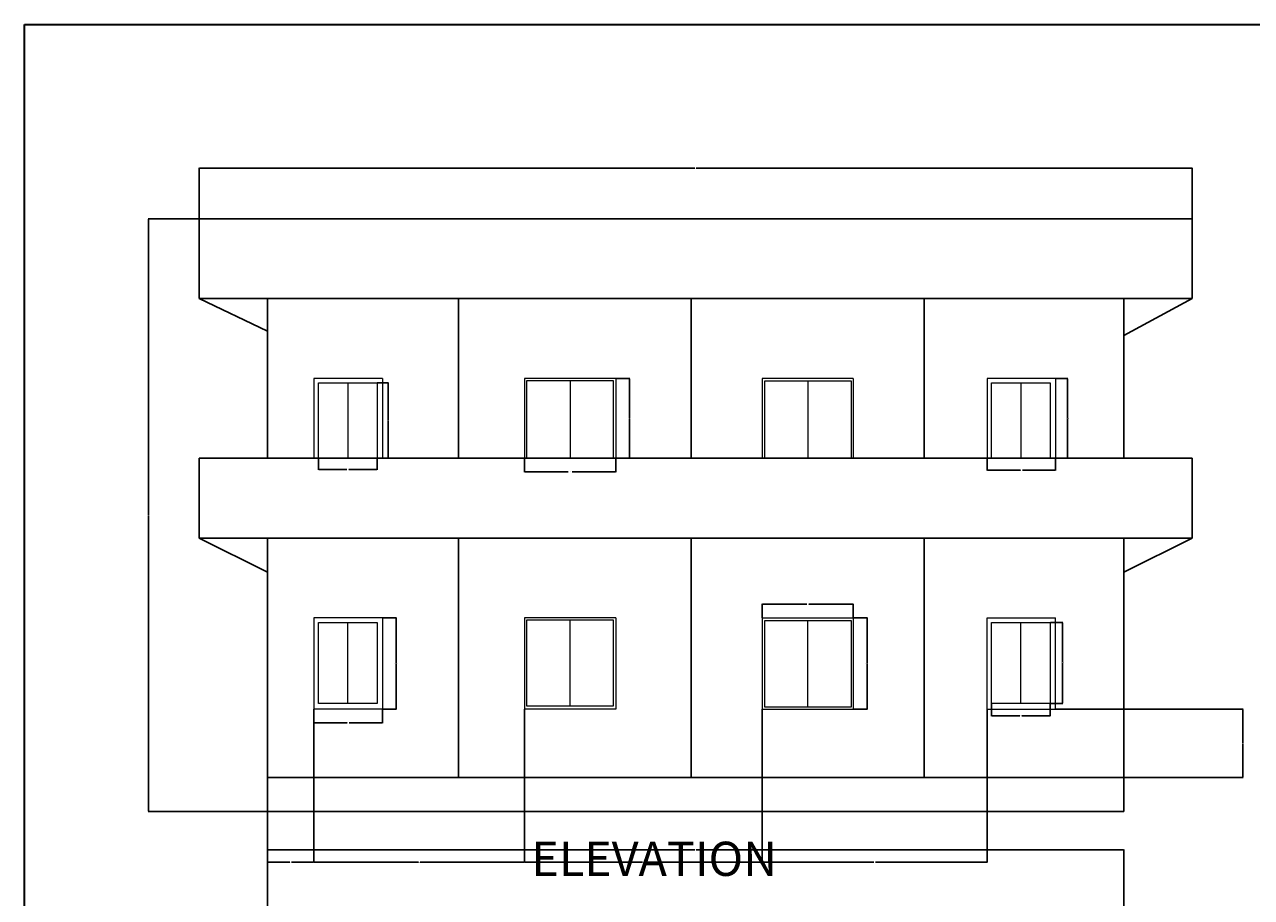
# Model space of a CAD drawing. Units: inches. Extents: x 2043 to 3387, y 1535 to 2797.
# Tile 3 of 7: x 2043 to 2688, y 2337 to 2797. Entities that reach past the tile are written whole.
import ezdxf

# ---------------------------------------------------------------- set-up
doc = ezdxf.new("R2010")
doc.units = ezdxf.units.IN
for name, color, linetype, lineweight in [('A-ANNO-DIMS', 2, 'Continuous', 18), ('A-ANNO-TITL', 7, 'Continuous', 30), ('A-ANNO-TTLB', 7, 'Continuous', 35), ('A-ELEV', 7, 'Continuous', 30), ('A-GLAZ', 4, 'Continuous', 18)]:
    doc.layers.add(name, color=color, linetype=linetype, lineweight=lineweight)
doc.styles.get("Standard").update_dxf_attribs({"font": 'arial.ttf'})
doc.dimstyles.get("Standard").update_dxf_attribs({"dimtxt": 0.18, "dimasz": 0.18, "dimexe": 0.18, "dimexo": 0.0625, "dimgap": 0.09, "dimtad": 0, "dimtih": 1, "dimtoh": 1, "dimdec": 4, "dimzin": 0, "dimdsep": 46, "dimtxsty": 'Standard', "dimcen": 0.09, "dimadec": 0, "dimazin": 0, "dimtfac": 1, "dimtdec": 4, "dimtofl": 0, "dimtmove": 0, "dimatfit": 3, "dimfxl": 1, "dimtolj": 1, "dimtzin": 0, "dimarcsym": 0})

# ---------------------------------------------------------------- blocks, each defined once
blk = doc.blocks.new('WINDOW-CASING-36-FULL')
for p, q in [((0, 48), (0, 0)), ((36, 48), (0, 48)), ((36, 48), (36, 0)), ((36, 0), (0, 0))]:
    blk.add_line(p, q)
blk = doc.blocks.new('WINDOW-CASING-36-UPPER')
for p, q in [((0, 42), (0, 0)), ((36, 42), (0, 42)), ((0, 42), (0, 0)), ((36, 42), (0, 42)), ((36, 42), (36, 0)), ((36, 42), (36, 0))]:
    blk.add_line(p, q)
blk = doc.blocks.new('WINDOW-CASING-48-FULL')
for p, q in [((0, 48), (0, 0)), ((48, 48), (0, 48)), ((48, 48), (48, 0)), ((48, 0), (0, 0))]:
    blk.add_line(p, q)
blk = doc.blocks.new('WINDOW-CASING-48-UPPER')
for p, q in [((0, 42), (0, 0)), ((48, 42), (0, 42)), ((0, 42), (0, 0)), ((48, 42), (0, 42)), ((48, 42), (48, 0)), ((48, 42), (48, 0))]:
    blk.add_line(p, q)
blk = doc.blocks.new('WINDOW-SASH-36-FULL')
blk.add_line((15.4, 0), (15.4, 42.69))
blk.add_lwpolyline([(0, 42.69), (30.81, 42.69), (30.81, 0), (0, 0)], close=True)
blk = doc.blocks.new('WINDOW-SASH-36-UPPER')
blk.add_line((15.4, 39.6), (15.4, 0))
blk.add_lwpolyline([(0, 0), (0, 39.6), (30.81, 39.6), (30.81, 0)])
blk = doc.blocks.new('*D91')
at = {"layer": 'A-ANNO-DIMS', "color": 0, "lineweight": -2, "transparency": 16777216}
for p, q in [((2230.88, 2484.55), (2238.19, 2484.55)), ((2238.01, 2484.37), (2238.01, 2460.73)), ((2238.01, 2436.73), (2238.01, 2460.37)), ((2230.88, 2436.55), (2238.19, 2436.55))]:
    blk.add_line(p, q, dxfattribs=at)
at = {"layer": 'A-ANNO-DIMS', "color": 0, "transparency": 16777216}
for points in [[(2237.98, 2484.37), (2238.04, 2484.37), (2238.01, 2484.55)], [(2237.98, 2436.73), (2238.04, 2436.73), (2238.01, 2436.55)]]:
    blk.add_solid(points, dxfattribs=at)
at = {"layer": 'Defpoints', "color": 0, "transparency": 16777216}
for p in [(2230.81, 2484.55), (2238.01, 2484.55), (2230.81, 2436.55)]:
    blk.add_point(p, dxfattribs=at)
at = {"layer": 'A-ANNO-DIMS', "color": 0, "transparency": 16777216, "insert": (2238.01, 2460.55), "char_height": 0.18, "attachment_point": 5}
blk.add_mtext('\\A1;CASING 48 TYP.', dxfattribs=at)
blk = doc.blocks.new('*D92')
at = {"layer": 'A-ANNO-DIMS', "color": 0, "lineweight": -2, "transparency": 16777216}
for p, q in [((2194.81, 2436.49), (2194.81, 2429.17)), ((2230.81, 2436.49), (2230.81, 2429.17)), ((2194.99, 2429.35), (2212.29, 2429.35)), ((2230.63, 2429.35), (2213.34, 2429.35))]:
    blk.add_line(p, q, dxfattribs=at)
at = {"layer": 'A-ANNO-DIMS', "color": 0, "transparency": 16777216}
for points in [[(2194.99, 2429.38), (2194.99, 2429.32), (2194.81, 2429.35)], [(2230.63, 2429.38), (2230.63, 2429.32), (2230.81, 2429.35)]]:
    blk.add_solid(points, dxfattribs=at)
at = {"layer": 'Defpoints', "color": 0, "transparency": 16777216}
for p in [(2194.81, 2436.55), (2230.81, 2436.55), (2230.81, 2429.35)]:
    blk.add_point(p, dxfattribs=at)
at = {"layer": 'A-ANNO-DIMS', "color": 0, "transparency": 16777216, "insert": (2212.81, 2429.35), "char_height": 0.18, "attachment_point": 5}
blk.add_mtext('\\A1;36 TYP.', dxfattribs=at)
blk = doc.blocks.new('*D93')
at = {"layer": 'A-ANNO-DIMS', "color": 0, "lineweight": -2, "transparency": 16777216}
for p, q in [((2585.12, 2610.55), (2591.53, 2610.55)), ((2591.35, 2610.37), (2591.35, 2589.73)), ((2591.35, 2568.73), (2591.35, 2589.37)), ((2585.12, 2568.55), (2591.53, 2568.55))]:
    blk.add_line(p, q, dxfattribs=at)
at = {"layer": 'A-ANNO-DIMS', "color": 0, "transparency": 16777216}
for points in [[(2591.32, 2610.37), (2591.38, 2610.37), (2591.35, 2610.55)], [(2591.32, 2568.73), (2591.38, 2568.73), (2591.35, 2568.55)]]:
    blk.add_solid(points, dxfattribs=at)
at = {"layer": 'Defpoints', "color": 0, "transparency": 16777216}
for p in [(2585.05, 2610.55), (2591.35, 2610.55), (2585.05, 2568.55)]:
    blk.add_point(p, dxfattribs=at)
at = {"layer": 'A-ANNO-DIMS', "color": 0, "transparency": 16777216, "insert": (2591.35, 2589.55), "char_height": 0.18, "attachment_point": 5}
blk.add_mtext('\\A1;CASING 42 TYP.', dxfattribs=at)
blk = doc.blocks.new('*D94')
at = {"layer": 'A-ANNO-DIMS', "color": 0, "lineweight": -2, "transparency": 16777216}
for p, q in [((2549.05, 2568.49), (2549.05, 2562.07)), ((2585.05, 2568.49), (2585.05, 2562.07)), ((2549.23, 2562.25), (2566.53, 2562.25)), ((2584.87, 2562.25), (2567.58, 2562.25))]:
    blk.add_line(p, q, dxfattribs=at)
at = {"layer": 'A-ANNO-DIMS', "color": 0, "transparency": 16777216}
for points in [[(2549.23, 2562.28), (2549.23, 2562.22), (2549.05, 2562.25)], [(2584.87, 2562.28), (2584.87, 2562.22), (2585.05, 2562.25)]]:
    blk.add_solid(points, dxfattribs=at)
at = {"layer": 'Defpoints', "color": 0, "transparency": 16777216}
for p in [(2549.05, 2568.55), (2585.05, 2568.55), (2585.05, 2562.25)]:
    blk.add_point(p, dxfattribs=at)
at = {"layer": 'A-ANNO-DIMS', "color": 0, "transparency": 16777216, "insert": (2567.05, 2562.25), "char_height": 0.18, "attachment_point": 5}
blk.add_mtext('\\A1;36 TYP.', dxfattribs=at)
blk = doc.blocks.new('*D95')
at = {"layer": 'A-ANNO-DIMS', "color": 0, "lineweight": -2, "transparency": 16777216}
for p, q in [((2478.66, 2484.55), (2485.98, 2484.55)), ((2485.8, 2484.37), (2485.8, 2460.73)), ((2485.8, 2436.73), (2485.8, 2460.37)), ((2478.66, 2436.55), (2485.98, 2436.55))]:
    blk.add_line(p, q, dxfattribs=at)
at = {"layer": 'A-ANNO-DIMS', "color": 0, "transparency": 16777216}
for points in [[(2485.77, 2484.37), (2485.83, 2484.37), (2485.8, 2484.55)], [(2485.77, 2436.73), (2485.83, 2436.73), (2485.8, 2436.55)]]:
    blk.add_solid(points, dxfattribs=at)
at = {"layer": 'Defpoints', "color": 0, "transparency": 16777216}
for p in [(2478.6, 2484.55), (2485.8, 2484.55), (2478.6, 2436.55)]:
    blk.add_point(p, dxfattribs=at)
at = {"layer": 'A-ANNO-DIMS', "color": 0, "transparency": 16777216, "insert": (2485.8, 2460.55), "char_height": 0.18, "attachment_point": 5}
blk.add_mtext('\\A1;CASING 48 TYP.', dxfattribs=at)
blk = doc.blocks.new('*D96')
at = {"layer": 'A-ANNO-DIMS', "color": 0, "lineweight": -2, "transparency": 16777216}
for p, q in [((2430.6, 2484.61), (2430.6, 2491.93)), ((2430.78, 2491.75), (2454.07, 2491.75)), ((2478.42, 2491.75), (2455.13, 2491.75)), ((2478.6, 2484.61), (2478.6, 2491.93))]:
    blk.add_line(p, q, dxfattribs=at)
at = {"layer": 'A-ANNO-DIMS', "color": 0, "transparency": 16777216}
for points in [[(2430.78, 2491.78), (2430.78, 2491.72), (2430.6, 2491.75)], [(2478.42, 2491.78), (2478.42, 2491.72), (2478.6, 2491.75)]]:
    blk.add_solid(points, dxfattribs=at)
at = {"layer": 'Defpoints', "color": 0, "transparency": 16777216}
for p in [(2430.6, 2491.75), (2430.6, 2484.55), (2478.6, 2484.55)]:
    blk.add_point(p, dxfattribs=at)
at = {"layer": 'A-ANNO-DIMS', "color": 0, "transparency": 16777216, "insert": (2454.6, 2491.75), "char_height": 0.18, "attachment_point": 5}
blk.add_mtext('\\A1;48 TYP.', dxfattribs=at)
blk = doc.blocks.new('*D97')
at = {"layer": 'A-ANNO-DIMS', "color": 0, "lineweight": -2, "transparency": 16777216}
for p, q in [((2305.57, 2568.49), (2305.57, 2561.17)), ((2353.57, 2568.49), (2353.57, 2561.17)), ((2305.75, 2561.35), (2328.53, 2561.35)), ((2353.39, 2561.35), (2330.61, 2561.35))]:
    blk.add_line(p, q, dxfattribs=at)
at = {"layer": 'A-ANNO-DIMS', "color": 0, "transparency": 16777216}
for points in [[(2305.75, 2561.38), (2305.75, 2561.32), (2305.57, 2561.35)], [(2353.39, 2561.38), (2353.39, 2561.32), (2353.57, 2561.35)]]:
    blk.add_solid(points, dxfattribs=at)
at = {"layer": 'Defpoints', "color": 0, "transparency": 16777216}
for p in [(2305.57, 2568.55), (2353.57, 2568.55), (2353.57, 2561.35)]:
    blk.add_point(p, dxfattribs=at)
at = {"layer": 'A-ANNO-DIMS', "color": 0, "transparency": 16777216, "insert": (2329.57, 2561.35), "char_height": 0.18, "attachment_point": 5}
blk.add_mtext('\\A1;CASING 48 TYP.', dxfattribs=at)
blk = doc.blocks.new('*D98')
at = {"layer": 'A-ANNO-DIMS', "color": 0, "lineweight": -2, "transparency": 16777216}
for p, q in [((2353.63, 2610.55), (2360.95, 2610.55)), ((2360.77, 2610.37), (2360.77, 2589.73)), ((2360.77, 2568.73), (2360.77, 2589.37)), ((2353.63, 2568.55), (2360.95, 2568.55))]:
    blk.add_line(p, q, dxfattribs=at)
at = {"layer": 'A-ANNO-DIMS', "color": 0, "transparency": 16777216}
for points in [[(2360.74, 2610.37), (2360.8, 2610.37), (2360.77, 2610.55)], [(2360.74, 2568.73), (2360.8, 2568.73), (2360.77, 2568.55)]]:
    blk.add_solid(points, dxfattribs=at)
at = {"layer": 'Defpoints', "color": 0, "transparency": 16777216}
for p in [(2353.57, 2610.55), (2360.77, 2610.55), (2353.57, 2568.55)]:
    blk.add_point(p, dxfattribs=at)
at = {"layer": 'A-ANNO-DIMS', "color": 0, "transparency": 16777216, "insert": (2360.77, 2589.55), "char_height": 0.18, "attachment_point": 5}
blk.add_mtext('\\A1;42 TYP.', dxfattribs=at)
blk = doc.blocks.new('*D99')
at = {"layer": 'A-ANNO-DIMS', "color": 0, "lineweight": -2, "transparency": 16777216}
for p, q in [((2582.25, 2482.15), (2588.77, 2482.15)), ((2588.59, 2481.97), (2588.59, 2460.99)), ((2588.59, 2439.64), (2588.59, 2460.62)), ((2582.25, 2439.46), (2588.77, 2439.46))]:
    blk.add_line(p, q, dxfattribs=at)
at = {"layer": 'A-ANNO-DIMS', "color": 0, "transparency": 16777216}
for points in [[(2588.56, 2481.97), (2588.62, 2481.97), (2588.59, 2482.15)], [(2588.56, 2439.64), (2588.62, 2439.64), (2588.59, 2439.46)]]:
    blk.add_solid(points, dxfattribs=at)
at = {"layer": 'Defpoints', "color": 0, "transparency": 16777216}
for p in [(2582.18, 2482.15), (2588.59, 2482.15), (2582.18, 2439.46)]:
    blk.add_point(p, dxfattribs=at)
at = {"layer": 'A-ANNO-DIMS', "color": 0, "transparency": 16777216, "insert": (2588.59, 2460.8), "char_height": 0.18, "attachment_point": 5}
blk.add_mtext('\\A1;SASH 43 TYP.', dxfattribs=at)
blk = doc.blocks.new('*D100')
at = {"layer": 'A-ANNO-DIMS', "color": 0, "lineweight": -2, "transparency": 16777216}
for p, q in [((2551.37, 2439.4), (2551.37, 2432.88)), ((2582.18, 2439.4), (2582.18, 2432.88)), ((2551.55, 2433.06), (2566.25, 2433.06)), ((2582, 2433.06), (2567.31, 2433.06))]:
    blk.add_line(p, q, dxfattribs=at)
at = {"layer": 'A-ANNO-DIMS', "color": 0, "transparency": 16777216}
for points in [[(2551.55, 2433.09), (2551.55, 2433.03), (2551.37, 2433.06)], [(2582, 2433.09), (2582, 2433.03), (2582.18, 2433.06)]]:
    blk.add_solid(points, dxfattribs=at)
at = {"layer": 'Defpoints', "color": 0, "transparency": 16777216}
for p in [(2551.37, 2439.46), (2582.18, 2439.46), (2582.18, 2433.06)]:
    blk.add_point(p, dxfattribs=at)
at = {"layer": 'A-ANNO-DIMS', "color": 0, "transparency": 16777216, "insert": (2566.78, 2433.06), "char_height": 0.18, "attachment_point": 5}
blk.add_mtext('\\A1;31 TYP.', dxfattribs=at)
blk = doc.blocks.new('*D101')
at = {"layer": 'A-ANNO-DIMS', "color": 0, "lineweight": -2, "transparency": 16777216}
for p, q in [((2228.07, 2608.15), (2234.13, 2608.15)), ((2233.95, 2607.97), (2233.95, 2588.53)), ((2233.95, 2568.73), (2233.95, 2588.17)), ((2228.07, 2568.55), (2234.13, 2568.55))]:
    blk.add_line(p, q, dxfattribs=at)
at = {"layer": 'A-ANNO-DIMS', "color": 0, "transparency": 16777216}
for points in [[(2233.92, 2607.97), (2233.98, 2607.97), (2233.95, 2608.15)], [(2233.92, 2568.73), (2233.98, 2568.73), (2233.95, 2568.55)]]:
    blk.add_solid(points, dxfattribs=at)
at = {"layer": 'Defpoints', "color": 0, "transparency": 16777216}
for p in [(2228.01, 2608.15), (2233.95, 2608.15), (2228.01, 2568.55)]:
    blk.add_point(p, dxfattribs=at)
at = {"layer": 'A-ANNO-DIMS', "color": 0, "transparency": 16777216, "insert": (2233.95, 2588.35), "char_height": 0.18, "attachment_point": 5}
blk.add_mtext('\\A1;SASH 40 TYP.', dxfattribs=at)
blk = doc.blocks.new('*D102')
at = {"layer": 'A-ANNO-DIMS', "color": 0, "lineweight": -2, "transparency": 16777216}
for p, q in [((2197.2, 2568.49), (2197.2, 2562.43)), ((2228.01, 2568.49), (2228.01, 2562.43)), ((2197.38, 2562.61), (2212.08, 2562.61)), ((2227.83, 2562.61), (2213.13, 2562.61))]:
    blk.add_line(p, q, dxfattribs=at)
at = {"layer": 'A-ANNO-DIMS', "color": 0, "transparency": 16777216}
for points in [[(2197.38, 2562.64), (2197.38, 2562.58), (2197.2, 2562.61)], [(2227.83, 2562.64), (2227.83, 2562.58), (2228.01, 2562.61)]]:
    blk.add_solid(points, dxfattribs=at)
at = {"layer": 'Defpoints', "color": 0, "transparency": 16777216}
for p in [(2197.2, 2568.55), (2228.01, 2568.55), (2228.01, 2562.61)]:
    blk.add_point(p, dxfattribs=at)
at = {"layer": 'A-ANNO-DIMS', "color": 0, "transparency": 16777216, "insert": (2212.6, 2562.61), "char_height": 0.18, "attachment_point": 5}
blk.add_mtext('\\A1;31 TYP.', dxfattribs=at)
blk = doc.blocks.new('*D103')
at = {"layer": 'A-ANNO-DIMS', "color": 0, "lineweight": -2, "transparency": 16777216}
for p, q in [((2170.35, 2326.44), (2170.35, 2362.56)), ((2170.53, 2362.38), (2395.2, 2362.38)), ((2620.67, 2362.38), (2396, 2362.38)), ((2620.85, 2326.44), (2620.85, 2362.56))]:
    blk.add_line(p, q, dxfattribs=at)
at = {"layer": 'A-ANNO-DIMS', "color": 0, "transparency": 16777216}
for points in [[(2170.53, 2362.41), (2170.53, 2362.35), (2170.35, 2362.38)], [(2620.67, 2362.41), (2620.67, 2362.35), (2620.85, 2362.38)]]:
    blk.add_solid(points, dxfattribs=at)
at = {"layer": 'Defpoints', "color": 0, "transparency": 16777216}
for p in [(2620.85, 2362.38), (2170.35, 2326.38), (2620.85, 2326.38)]:
    blk.add_point(p, dxfattribs=at)
at = {"layer": 'A-ANNO-DIMS', "color": 0, "transparency": 16777216, "insert": (2395.6, 2362.38), "char_height": 0.18, "attachment_point": 5}
blk.add_mtext('\\A1;450.5', dxfattribs=at)
blk = doc.blocks.new('*D118')
at = {"layer": 'A-ANNO-DIMS', "color": 0, "lineweight": -2, "transparency": 16777216}
for p, q in [((2134.35, 2694.61), (2134.35, 2721.38)), ((2134.53, 2721.2), (2395.21, 2721.2)), ((2656.67, 2721.2), (2395.99, 2721.2)), ((2656.85, 2694.61), (2656.85, 2721.38))]:
    blk.add_line(p, q, dxfattribs=at)
at = {"layer": 'A-ANNO-DIMS', "color": 0, "transparency": 16777216}
for points in [[(2134.53, 2721.23), (2134.53, 2721.17), (2134.35, 2721.2)], [(2656.67, 2721.23), (2656.67, 2721.17), (2656.85, 2721.2)]]:
    blk.add_solid(points, dxfattribs=at)
at = {"layer": 'Defpoints', "color": 0, "transparency": 16777216}
for p in [(2656.85, 2721.2), (2134.35, 2694.55), (2656.85, 2694.55)]:
    blk.add_point(p, dxfattribs=at)
at = {"layer": 'A-ANNO-DIMS', "color": 0, "transparency": 16777216, "insert": (2395.6, 2721.2), "char_height": 0.18, "attachment_point": 5}
blk.add_mtext('\\A1;522.5', dxfattribs=at)
blk = doc.blocks.new('*D119')
at = {"layer": 'A-ANNO-DIMS', "color": 0, "lineweight": -2, "transparency": 16777216}
for p, q in [((2134.29, 2694.55), (2107.52, 2694.55)), ((2107.7, 2694.37), (2107.7, 2538.73)), ((2107.7, 2382.73), (2107.7, 2538.37)), ((2170.29, 2382.55), (2107.52, 2382.55))]:
    blk.add_line(p, q, dxfattribs=at)
at = {"layer": 'A-ANNO-DIMS', "color": 0, "transparency": 16777216}
for points in [[(2107.67, 2694.37), (2107.73, 2694.37), (2107.7, 2694.55)], [(2107.67, 2382.73), (2107.73, 2382.73), (2107.7, 2382.55)]]:
    blk.add_solid(points, dxfattribs=at)
at = {"layer": 'Defpoints', "color": 0, "transparency": 16777216}
for p in [(2107.7, 2694.55), (2134.35, 2694.55), (2170.35, 2382.55)]:
    blk.add_point(p, dxfattribs=at)
at = {"layer": 'A-ANNO-DIMS', "color": 0, "transparency": 16777216, "insert": (2107.7, 2538.55), "char_height": 0.18, "attachment_point": 5}
blk.add_mtext('\\A1;312', dxfattribs=at)
blk = doc.blocks.new('*D122')
at = {"layer": 'A-ANNO-DIMS', "color": 0, "lineweight": -2, "transparency": 16777216}
for p, q in [((2194.81, 2436.49), (2194.81, 2355.72)), ((2170.35, 2400.49), (2170.35, 2355.72)), ((2170.53, 2355.9), (2182.12, 2355.9)), ((2194.63, 2355.9), (2183.05, 2355.9))]:
    blk.add_line(p, q, dxfattribs=at)
at = {"layer": 'A-ANNO-DIMS', "color": 0, "transparency": 16777216}
for points in [[(2170.53, 2355.93), (2170.53, 2355.87), (2170.35, 2355.9)], [(2194.63, 2355.93), (2194.63, 2355.87), (2194.81, 2355.9)]]:
    blk.add_solid(points, dxfattribs=at)
at = {"layer": 'Defpoints', "color": 0, "transparency": 16777216}
for p in [(2194.81, 2436.55), (2170.35, 2400.55), (2194.81, 2355.9)]:
    blk.add_point(p, dxfattribs=at)
at = {"layer": 'A-ANNO-DIMS', "color": 0, "transparency": 16777216, "insert": (2182.58, 2355.9), "char_height": 0.18, "attachment_point": 5}
blk.add_mtext('\\A1;24.464', dxfattribs=at)
blk = doc.blocks.new('*D123')
at = {"layer": 'A-ANNO-DIMS', "color": 0, "lineweight": -2, "transparency": 16777216}
for p, q in [((2194.81, 2436.49), (2194.81, 2355.72)), ((2305.57, 2436.49), (2305.57, 2355.72)), ((2194.99, 2355.9), (2249.74, 2355.9)), ((2305.39, 2355.9), (2250.65, 2355.9))]:
    blk.add_line(p, q, dxfattribs=at)
at = {"layer": 'A-ANNO-DIMS', "color": 0, "transparency": 16777216}
for points in [[(2194.99, 2355.93), (2194.99, 2355.87), (2194.81, 2355.9)], [(2305.39, 2355.93), (2305.39, 2355.87), (2305.57, 2355.9)]]:
    blk.add_solid(points, dxfattribs=at)
at = {"layer": 'Defpoints', "color": 0, "transparency": 16777216}
for p in [(2194.81, 2436.55), (2305.57, 2436.55), (2305.57, 2355.9)]:
    blk.add_point(p, dxfattribs=at)
at = {"layer": 'A-ANNO-DIMS', "color": 0, "transparency": 16777216, "insert": (2250.19, 2355.9), "char_height": 0.18, "attachment_point": 5}
blk.add_mtext('\\A1;110.76', dxfattribs=at)
blk = doc.blocks.new('*D124')
at = {"layer": 'A-ANNO-DIMS', "color": 0, "lineweight": -2, "transparency": 16777216}
for p, q in [((2305.57, 2436.49), (2305.57, 2355.72)), ((2430.6, 2436.49), (2430.6, 2355.72)), ((2305.75, 2355.9), (2367.63, 2355.9)), ((2430.42, 2355.9), (2368.54, 2355.9))]:
    blk.add_line(p, q, dxfattribs=at)
at = {"layer": 'A-ANNO-DIMS', "color": 0, "transparency": 16777216}
for points in [[(2305.75, 2355.93), (2305.75, 2355.87), (2305.57, 2355.9)], [(2430.42, 2355.93), (2430.42, 2355.87), (2430.6, 2355.9)]]:
    blk.add_solid(points, dxfattribs=at)
at = {"layer": 'Defpoints', "color": 0, "transparency": 16777216}
for p in [(2305.57, 2436.55), (2430.6, 2436.55), (2430.6, 2355.9)]:
    blk.add_point(p, dxfattribs=at)
at = {"layer": 'A-ANNO-DIMS', "color": 0, "transparency": 16777216, "insert": (2368.08, 2355.9), "char_height": 0.18, "attachment_point": 5}
blk.add_mtext('\\A1;125.03', dxfattribs=at)
blk = doc.blocks.new('*D125')
at = {"layer": 'A-ANNO-DIMS', "color": 0, "lineweight": -2, "transparency": 16777216}
for p, q in [((2430.6, 2436.49), (2430.6, 2355.72)), ((2549.05, 2436.49), (2549.05, 2355.72)), ((2430.78, 2355.9), (2489.37, 2355.9)), ((2548.87, 2355.9), (2490.28, 2355.9))]:
    blk.add_line(p, q, dxfattribs=at)
at = {"layer": 'A-ANNO-DIMS', "color": 0, "transparency": 16777216}
for points in [[(2430.78, 2355.93), (2430.78, 2355.87), (2430.6, 2355.9)], [(2548.87, 2355.93), (2548.87, 2355.87), (2549.05, 2355.9)]]:
    blk.add_solid(points, dxfattribs=at)
at = {"layer": 'Defpoints', "color": 0, "transparency": 16777216}
for p in [(2430.6, 2436.55), (2549.05, 2436.55), (2549.05, 2355.9)]:
    blk.add_point(p, dxfattribs=at)
at = {"layer": 'A-ANNO-DIMS', "color": 0, "transparency": 16777216, "insert": (2489.83, 2355.9), "char_height": 0.18, "attachment_point": 5}
blk.add_mtext('\\A1;118.45', dxfattribs=at)
blk = doc.blocks.new('*D126')
at = {"layer": 'A-ANNO-DIMS', "color": 0, "lineweight": -2, "transparency": 16777216}
for p, q in [((2585.12, 2436.55), (2683.68, 2436.55)), ((2683.5, 2436.37), (2683.5, 2418.73)), ((2683.5, 2400.73), (2683.5, 2418.37)), ((2620.91, 2400.55), (2683.68, 2400.55))]:
    blk.add_line(p, q, dxfattribs=at)
at = {"layer": 'A-ANNO-DIMS', "color": 0, "transparency": 16777216}
for points in [[(2683.47, 2436.37), (2683.53, 2436.37), (2683.5, 2436.55)], [(2683.47, 2400.73), (2683.53, 2400.73), (2683.5, 2400.55)]]:
    blk.add_solid(points, dxfattribs=at)
at = {"layer": 'Defpoints', "color": 0, "transparency": 16777216}
for p in [(2585.05, 2436.55), (2683.5, 2436.55), (2620.85, 2400.55)]:
    blk.add_point(p, dxfattribs=at)
at = {"layer": 'A-ANNO-DIMS', "color": 0, "transparency": 16777216, "insert": (2683.5, 2418.55), "char_height": 0.18, "attachment_point": 5}
blk.add_mtext('\\A1;36', dxfattribs=at)

msp = doc.modelspace()

# ---------------------------------------------------------------- linework, layer by layer
at = {"layer": 'A-ANNO-TTLB'}
msp.add_lwpolyline([(2042.5541, 2796.7818), (3386.9704, 2796.7818), (3386.9704, 1534.5689), (2042.5541, 1534.5689)], close=True, dxfattribs=at)
at = {"layer": 'A-ELEV'}
for p, q in [((2656.8496, 2694.549), (2134.3496, 2694.549)), ((2134.3496, 2652.549), (2134.3496, 2694.549)), ((2656.8496, 2652.549), (2656.8496, 2694.549)), ((2656.8496, 2652.549), (2134.3496, 2652.549)), ((2134.3496, 2652.549), (2170.3496, 2635.4793)), ((2170.3496, 2652.549), (2170.3496, 2568.549)), ((2270.8496, 2568.549), (2270.8496, 2652.549)), ((2393.3496, 2568.549), (2393.3496, 2652.549)), ((2515.8496, 2568.549), (2515.8496, 2652.549)), ((2620.8496, 2652.549), (2620.8496, 2568.549)), ((2656.8496, 2652.549), (2620.8496, 2633.1824)), ((2656.8496, 2568.549), (2134.3496, 2568.549)), ((2134.3496, 2526.549), (2134.3496, 2568.549)), ((2656.8496, 2526.549), (2656.8496, 2568.549)), ((2656.8496, 2526.549), (2134.3496, 2526.549)), ((2134.3496, 2526.549), (2134.3496, 2526.549)), ((2134.3496, 2526.549), (2170.3496, 2508.549)), ((2170.3496, 2526.549), (2170.3496, 2382.549)), ((2170.3496, 2526.549), (2170.3496, 2508.549)), ((2270.8496, 2400.549), (2270.8496, 2526.549)), ((2393.3496, 2400.549), (2393.3496, 2526.549)), ((2515.8496, 2400.549), (2515.8496, 2526.549)), ((2620.8496, 2526.549), (2620.8496, 2382.549)), ((2620.8496, 2526.549), (2620.8496, 2508.549)), ((2656.8496, 2526.549), (2620.8496, 2508.549)), ((2620.8496, 2400.549), (2170.3496, 2400.549)), ((2620.8496, 2382.549), (2170.3496, 2382.549))]:
    msp.add_line(p, q, dxfattribs=at)
at = {"layer": 'A-GLAZ'}
for p, q in [((2329.5531, 2609.485), (2329.5531, 2568.549)), ((2454.736, 2609.217), (2454.736, 2568.549)), ((2329.5531, 2438.0168), (2329.5531, 2483.485)), ((2454.736, 2437.4983), (2454.736, 2483.217))]:
    msp.add_line(p, q, dxfattribs=at)
for points in [[(2306.8471, 2568.549), (2306.8471, 2609.485), (2352.2592, 2609.485), (2352.2592, 2568.549)], [(2431.9792, 2568.549), (2431.9792, 2609.217), (2477.4928, 2609.217), (2477.4928, 2568.549)]]:
    msp.add_lwpolyline(points, dxfattribs=at)
for points in [[(2306.8471, 2483.485), (2352.2592, 2483.485), (2352.2592, 2438.0168), (2306.8471, 2438.0168)], [(2431.9792, 2483.217), (2477.4928, 2483.217), (2477.4928, 2437.4983), (2431.9792, 2437.4983)]]:
    msp.add_lwpolyline(points, close=True, dxfattribs=at)

# ---------------------------------------------------------------- block references
for name, p in [('WINDOW-CASING-36-UPPER', (2194.813, 2568.549)), ('WINDOW-SASH-36-UPPER', (2197.199, 2568.549)), ('WINDOW-CASING-48-UPPER', (2305.57, 2568.549)), ('WINDOW-CASING-48-UPPER', (2430.5985, 2568.549)), ('WINDOW-CASING-36-UPPER', (2549.0536, 2568.549)), ('WINDOW-SASH-36-UPPER', (2551.3743, 2568.549)), ('WINDOW-CASING-36-FULL', (2194.813, 2436.549)), ('WINDOW-SASH-36-FULL', (2197.199, 2439.462)), ('WINDOW-CASING-48-FULL', (2305.57, 2436.549)), ('WINDOW-SASH-36-FULL', (2551.3743, 2439.462))]:
    msp.add_blockref(name, p, dxfattribs=at)
for name, p, rotation in [('WINDOW-CASING-48-FULL', (2478.5989, 2436.5485), 89.9999999999989), ('WINDOW-CASING-36-FULL', (2585.0542, 2484.5489), 180)]:
    msp.add_blockref(name, p, dxfattribs=dict(at, rotation=rotation))

# ---------------------------------------------------------------- texts
at = {"layer": 'A-ANNO-TITL', "insert": (2309.2082, 2366.7325), "char_height": 18, "attachment_point": 1}
msp.add_mtext_dynamic_manual_height_columns('ELEVATION', width=215.826045, gutter_width=12.5, heights=[0], dxfattribs=at)

# ---------------------------------------------------------------- dimensions: what is measured, and where the dimension line sits
at = {"layer": 'A-ANNO-DIMS'}
for base, p1, p2, override, picture, middle in [((2656.8496, 2721.199), (2134.3496, 2694.549), (2656.8496, 2694.549), {"dimdec": 1, "dimlfac": 1, "dimrnd": 0, "dimzin": 0, "dimdsep": 46, "dimlunit": 2}, '*D118', (2395.5996, 2721.199)), ((2194.8133, 2355.899), (2170.3496, 2400.549), (2194.8133, 2436.549), {"dimdec": 3, "dimlfac": 1, "dimrnd": 0, "dimzin": 0, "dimdsep": 46, "dimlunit": 2}, '*D122', (2182.5815, 2355.899)), ((2305.5704, 2355.899), (2194.8133, 2436.549), (2305.5704, 2436.549), {"dimdec": 2, "dimlfac": 1, "dimrnd": 0, "dimzin": 0, "dimdsep": 46, "dimlunit": 2}, '*D123', (2250.1919, 2355.899)), ((2430.5989, 2355.899), (2305.5704, 2436.549), (2430.5989, 2436.549), {"dimdec": 2, "dimlfac": 1, "dimrnd": 0, "dimzin": 0, "dimdsep": 46, "dimlunit": 2}, '*D124', (2368.0847, 2355.899)), ((2549.05389, 2355.89895), (2430.59895, 2436.54895), (2549.05389, 2436.54895), {"dimdec": 2, "dimlfac": 1, "dimrnd": 0, "dimzin": 0, "dimdsep": 46, "dimlunit": 2}, '*D125', (2489.82642, 2355.89895)), ((2620.8496, 2362.3769), (2170.3496, 2326.3769), (2620.8496, 2326.3769), {"dimdec": 1, "dimlfac": 1, "dimrnd": 0, "dimzin": 0, "dimdsep": 46, "dimlunit": 2}, '*D103', (2395.5996, 2362.3769))]:
    dim = msp.add_linear_dim(base=base, p1=p1, p2=p2, dimstyle='Standard', override=override, dxfattribs=at)
    dim.commit()
    dim.dimension.update_dxf_attribs({"geometry": picture, "text_midpoint": middle})
for base, p1, p2, picture, middle in [((2107.6996, 2694.549), (2170.3496, 2382.549), (2134.3496, 2694.549), '*D119', (2107.6996, 2538.549)), ((2683.4996, 2436.549), (2620.8496, 2400.549), (2585.0539, 2436.549), '*D126', (2683.4996, 2418.549))]:
    dim = msp.add_linear_dim(base=base, p1=p1, p2=p2, angle=90, dimstyle='Standard', override={"dimdec": 0, "dimlfac": 1, "dimrnd": 0, "dimzin": 0, "dimdsep": 46, "dimlunit": 2}, dxfattribs=at)
    dim.commit()
    dim.dimension.update_dxf_attribs({"geometry": picture, "text_midpoint": middle})
for base, p1, p2, angle, text, picture, middle in [((2233.948, 2608.1477), (2228.0082, 2568.549), (2228.0082, 2608.1477), 90, 'SASH <> TYP.', '*D101', (2233.948, 2588.3483)), ((2360.7704, 2610.549), (2353.5704, 2568.549), (2353.5704, 2610.549), 90, '<> TYP.', '*D98', (2360.7704, 2589.549)), ((2591.3539, 2610.549), (2585.0539, 2568.549), (2585.0539, 2610.549), 90, 'CASING <> TYP.', '*D93', (2591.3539, 2589.549)), ((2430.5989, 2491.749), (2478.5989, 2484.549), (2430.5989, 2484.549), 180, '<> TYP.', '*D96', (2454.5989, 2491.749)), ((2238.0133, 2484.549), (2230.8133, 2436.549), (2230.8133, 2484.549), 90, 'CASING <> TYP.', '*D91', (2238.0133, 2460.549)), ((2485.7989, 2484.549), (2478.5989, 2436.549), (2478.5989, 2484.549), 90, 'CASING <> TYP.', '*D95', (2485.7989, 2460.549)), ((2588.5863, 2482.1477), (2582.1834, 2439.4619), (2582.1834, 2482.1477), 90, 'SASH <> TYP.', '*D99', (2588.5863, 2460.8048))]:
    dim = msp.add_linear_dim(base=base, p1=p1, p2=p2, angle=angle, text=text, dimstyle='Standard', override={"dimdec": 0, "dimlfac": 1, "dimrnd": 0, "dimzin": 0, "dimdsep": 46, "dimlunit": 2}, dxfattribs=at)
    dim.commit()
    dim.dimension.update_dxf_attribs({"geometry": picture, "text_midpoint": middle})
for base, p1, p2, text, picture, middle in [((2228.0082, 2562.6091), (2197.1989, 2568.549), (2228.0082, 2568.549), '<> TYP.', '*D102', (2212.6035, 2562.6091)), ((2353.5704, 2561.349), (2305.5704, 2568.549), (2353.5704, 2568.549), 'CASING <> TYP.', '*D97', (2329.5704, 2561.349)), ((2585.0539, 2562.249), (2549.0539, 2568.549), (2585.0539, 2568.549), '<> TYP.', '*D94', (2567.0539, 2562.249)), ((2230.8133, 2429.349), (2194.8133, 2436.549), (2230.8133, 2436.549), '<> TYP.', '*D92', (2212.8133, 2429.349)), ((2582.1834, 2433.0591), (2551.3742, 2439.4619), (2582.1834, 2439.4619), '<> TYP.', '*D100', (2566.7788, 2433.0591))]:
    dim = msp.add_linear_dim(base=base, p1=p1, p2=p2, text=text, dimstyle='Standard', override={"dimdec": 0, "dimlfac": 1, "dimrnd": 0, "dimzin": 0, "dimdsep": 46, "dimlunit": 2}, dxfattribs=at)
    dim.commit()
    dim.dimension.update_dxf_attribs({"geometry": picture, "text_midpoint": middle})

doc.saveas('drawing.dxf')
